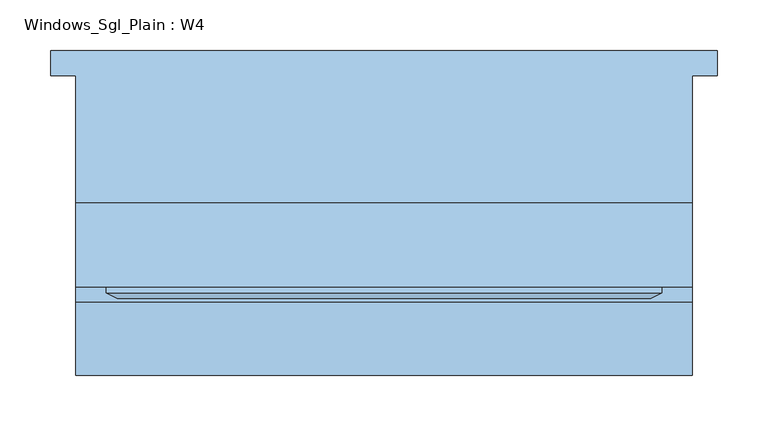
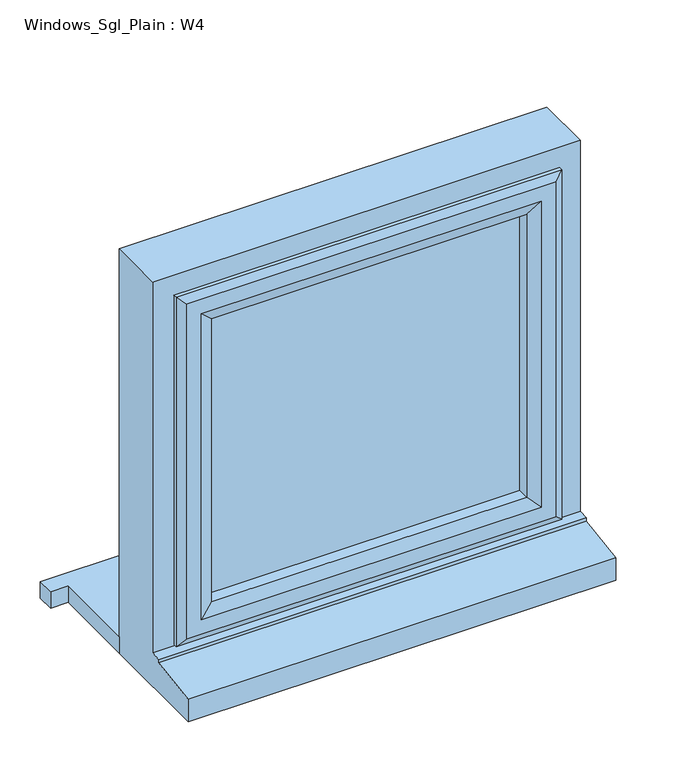
"""IFC4 building model written with IfcOpenShell, lengths in millimetres: window geometry, Windows_Sgl_Plain : W4."""

from ifc_helpers import new_model, si_unit, frame, origin, place, context, project, spatial, polyline, outline, extrude, faceted_brep, source, transform, mapped, element, save


def windows_sgl_plain_w4_0cd65ee0(model_context):
    return source(origin(), model_context, "Body", "SolidModel", [
        extrude(outline(polyline([(-329.8, 146.0834322), (329.8, 146.0834322), (329.8, 121.0834322), (304.8, 121.0834322), (304.8, -4.9965678), (-304.8, -4.9965678), (-304.8, 121.0834322), (-329.8, 121.0834322), (-329.8, 146.0834322)])), frame((0.0, 0.0, 1500.4), z_axis=(0.0, 0.0, 1.0), x_axis=(1.0, 0.0, 0.0)), (0.0, 0.0, 1.0), 25.0),
        faceted_brep([(-304.8, -4.9965678, 1500.4), (-304.8, -4.9965678, 2110.0), (304.8, -4.9965678, 2110.0), (304.8, -4.9965678, 1500.4), (-244.8, -4.9965678, 2050.0), (-244.8, -4.9965678, 1575.4), (244.8, -4.9965678, 1575.4), (244.8, -4.9965678, 2050.0), (-304.8, -175.4965678, 1500.4), (-304.8, -175.4965678, 1534.2088847), (-304.8, -102.9965678, 1545.1449676), (-304.8, -102.9965678, 1550.08767), (-304.8, -87.9965678, 1551.4), (-304.8, -87.9965678, 2110.0), (304.8, -87.9965678, 1551.4), (304.8, -87.9965678, 2110.0), (-264.8, -87.9965678, 2070.0), (264.8, -87.9965678, 2070.0), (264.8, -87.9965678, 1563.4), (-264.8, -87.9965678, 1563.4), (-264.8, -22.9965678, 1563.4), (-264.8, -22.9965678, 2070.0), (264.8, -22.9965678, 1563.4), (264.8, -22.9965678, 2070.0), (-244.8, -22.9965678, 2050.0), (244.8, -22.9965678, 2050.0), (244.8, -22.9965678, 1575.4), (-244.8, -22.9965678, 1575.4), (304.8, -102.9965678, 1550.08767), (304.8, -102.9965678, 1545.1449676), (304.8, -175.4965678, 1534.2088847), (304.8, -175.4965678, 1500.4)], [[[0, 1, 2, 3], [4, 5, 6, 7]], [[0, 8, 9, 10, 11, 12, 13, 1]], [[12, 14, 15, 13], [16, 17, 18, 19]], [[19, 20, 21, 16]], [[21, 20, 22, 23], [24, 25, 26, 27]], [[24, 27, 5, 4]], [[1, 13, 15, 2]], [[16, 21, 23, 17]], [[7, 25, 24, 4]], [[14, 28, 29, 30, 31, 3, 2, 15]], [[17, 23, 22, 18]], [[7, 6, 26, 25]], [[31, 8, 0, 3]], [[30, 9, 8, 31]], [[29, 10, 9, 30]], [[28, 11, 10, 29]], [[14, 12, 11, 28]], [[20, 19, 18, 22]], [[5, 27, 26, 6]]]),
        extrude(outline(polyline([(234.8, -51.9965678), (234.8, -75.9965678), (-234.8, -75.9965678), (-234.8, -51.9965678), (234.8, -51.9965678)])), frame((0.0, 0.0, 1593.4), z_axis=(0.0, 0.0, 1.0), x_axis=(1.0, 0.0, 0.0)), (0.0, 0.0, 1.0), 446.6),
        faceted_brep([(-274.8, -87.9965678, 2080.0), (-274.8, -87.9965678, 1553.4), (-274.8, -93.7700705, 1553.4), (-274.8, -93.7700705, 2080.0), (-264.8, -22.9965678, 2070.0), (-264.8, -22.9965678, 1563.4), (-264.8, -87.9965678, 1563.4), (-264.8, -87.9965678, 2070.0), (-224.8, -37.4894677, 2030.0), (-224.8, -37.4894677, 1603.4), (-234.9480377, -22.9965678, 1593.2519623), (-234.9480377, -22.9965678, 2040.1480377), (-224.8, -51.9965678, 2030.0), (-224.8, -51.9965678, 1603.4), (-234.8, -75.9965678, 2040.0), (-234.8, -75.9965678, 1593.4), (-234.8, -51.9965678, 1593.4), (-234.8, -51.9965678, 2040.0), (-224.8, -93.7700705, 2030.0), (-224.8, -93.7700705, 1603.4), (-224.8, -75.9965678, 1603.4), (-224.8, -75.9965678, 2030.0), (-242.2457548, -99.5435732, 2047.4457548), (-242.2457548, -99.5435732, 1585.9542452), (-264.0153903, -99.5435732, 1564.1846097), (-264.0153903, -99.5435732, 2069.2153903), (274.8, -87.9965678, 1553.4), (274.8, -93.7700705, 1553.4), (264.8, -22.9965678, 1563.4), (264.8, -87.9965678, 1563.4), (224.8, -37.4894677, 1603.4), (234.9480377, -22.9965678, 1593.2519623), (224.8, -51.9965678, 1603.4), (234.8, -75.9965678, 1593.4), (234.8, -51.9965678, 1593.4), (224.8, -93.7700705, 1603.4), (224.8, -75.9965678, 1603.4), (242.2457548, -99.5435732, 1585.9542452), (264.0153903, -99.5435732, 1564.1846097), (274.8, -87.9965678, 2080.0), (274.8, -93.7700705, 2080.0), (264.8, -22.9965678, 2070.0), (264.8, -87.9965678, 2070.0), (224.8, -37.4894677, 2030.0), (234.9480377, -22.9965678, 2040.1480377), (224.8, -51.9965678, 2030.0), (234.8, -75.9965678, 2040.0), (234.8, -51.9965678, 2040.0), (224.8, -93.7700705, 2030.0), (224.8, -75.9965678, 2030.0), (242.2457548, -99.5435732, 2047.4457548), (264.0153903, -99.5435732, 2069.2153903)], [[[0, 1, 2, 3]], [[4, 5, 6, 7]], [[8, 9, 10, 11]], [[12, 13, 9, 8]], [[14, 15, 16, 17]], [[18, 19, 20, 21]], [[22, 23, 19, 18]], [[3, 2, 24, 25]], [[1, 26, 27, 2]], [[5, 28, 29, 6]], [[9, 30, 31, 10]], [[13, 32, 30, 9]], [[15, 33, 34, 16]], [[19, 35, 36, 20]], [[23, 37, 35, 19]], [[2, 27, 38, 24]], [[26, 39, 40, 27]], [[28, 41, 42, 29]], [[30, 43, 44, 31]], [[32, 45, 43, 30]], [[33, 46, 47, 34]], [[35, 48, 49, 36]], [[37, 50, 48, 35]], [[27, 40, 51, 38]], [[39, 0, 3, 40]], [[1, 0, 39, 26], [7, 6, 29, 42]], [[41, 4, 7, 42]], [[5, 4, 41, 28], [11, 10, 31, 44]], [[43, 8, 11, 44]], [[45, 12, 8, 43]], [[17, 16, 34, 47], [13, 12, 45, 32]], [[46, 14, 17, 47]], [[15, 14, 46, 33], [21, 20, 36, 49]], [[48, 18, 21, 49]], [[50, 22, 18, 48]], [[25, 24, 38, 51], [23, 22, 50, 37]], [[40, 3, 25, 51]]]),
    ])


if __name__ == "__main__":
    model = new_model("IFC4")
    model_context = context("Model", 3, world=origin())
    ifc_project = project(units=[si_unit("LENGTHUNIT", "METRE", prefix="MILLI")], contexts=[model_context])
    site = spatial("IfcSite", under=ifc_project)
    building = spatial("IfcBuilding", under=site)
    placement = place(None, origin())
    windows_sgl_plain_w4_shape = windows_sgl_plain_w4_0cd65ee0(model_context)
    element("IfcWindow", 1, ObjectType="Windows_Sgl_Plain : W4", at=placement, inside=building, context=model_context, shape_type="MappedRepresentation", body=[
        mapped(windows_sgl_plain_w4_shape, transform((0.0, 0.0, 0.0), x_axis=(1.0, 0.0, 0.0), y_axis=(0.0, 1.0, 0.0), z_axis=(0.0, 0.0, 1.0))),
    ])
    save(model, "model.ifc")

# Revit data of these elements
# Type "Windows_Sgl_Plain : W4"
#   Type Mark = "59"
#   Operation = "SinglePanel"
#   Construction Type Id = "SGL"
#   Manufacturer = "Revit"
#   Keynote = "L10"
#   Analytic Construction = "Large single-glazed windows"
#   Wrap Layers (Ext) from Ext = 102.5 mm
#   Wrap Layers (Int) from Ext = 177.5 mm
#   Window Board Projection = 25 mm
#   Window Board Extension = 25 mm
#   Visual Light Transmittance = 0.9
#   Solar Heat Gain Coefficient = 0.86
#   Rough Width = 609.6 mm
#   Rough Height = 609.6 mm
#   Height = 609.6 mm
#   Width = 609.6 mm
#   Heat Transfer Coefficient (U) = 5.5617 W/(m²·K)
#   Glazing Thickness = 24 mm
#   FrameOffset - External = 50 mm
#   Frame Depth = 65 mm
#   Default Head Height = 2110 mm
#   Cill Depth = 87.5 mm
#   Cavity Closer Width = 50 mm
#   Cavity Closer Offset from Ext = 102.5 mm
#   Cavity Closer Depth = 85 mm
#   Vis - Cavity Closers = yes
#   Define Thermal Properties by = 1
#   Material Trim = Window Frame
#   Material Glass = Glass
#   Material Frame = Window Frame
#   Wall Closure = (empty or 0)
# Element 1 (IfcWindow, "Windows_Sgl_Plain : W4")
#   Materials on its faces: "Window Frame", "Glass"
# Materials
#   "Window Frame": colour RGB 249 249 249, transparency 0, Keynote = "L10", Cost = 0
#   "Glass": class "Glass", colour RGB 0 128 192, transparency 0.9, Description = "Soda Lime Glass", Cost = 0
